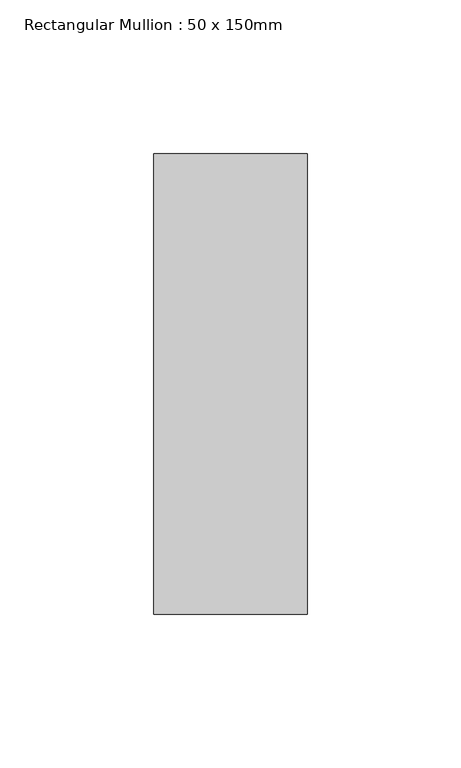
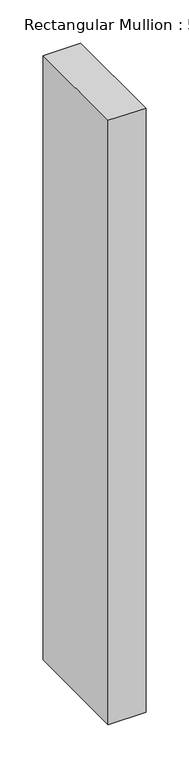
"""IFC4 building model written with IfcOpenShell, lengths in millimetres: member geometry, Rectangular Mullion : 50 x 150mm."""

from ifc_helpers import new_model, si_unit, frame, origin, place, context, project, spatial, polyline, outline, extrude, source, transform, mapped, element, save


def rectangular_mullion_50_x_150mm_324a6438(model_context):
    return source(origin(), model_context, "Body", "SweptSolid", [
        extrude(outline(polyline([(0.0, 75.0), (0.0, -75.0), (-50.0, -75.0), (-50.0, 75.0), (0.0, 75.0)])), frame((0.0, 0.0, -850.0), z_axis=(0.0, 0.0, 1.0), x_axis=(1.0, 0.0, 0.0)), (0.0, 0.0, 1.0), 850.0),
    ])


if __name__ == "__main__":
    model = new_model("IFC4")
    model_context = context("Model", 3, world=origin())
    ifc_project = project(units=[si_unit("LENGTHUNIT", "METRE", prefix="MILLI")], contexts=[model_context])
    site = spatial("IfcSite", under=ifc_project)
    building = spatial("IfcBuilding", under=site)
    placement = place(None, origin())
    rectangular_mullion_50_x_150mm_shape = rectangular_mullion_50_x_150mm_324a6438(model_context)
    element("IfcMember", 1, ObjectType="Rectangular Mullion : 50 x 150mm", at=placement, inside=building, context=model_context, shape_type="MappedRepresentation", body=[
        mapped(rectangular_mullion_50_x_150mm_shape, transform((0.0, 0.0, 0.0), x_axis=(1.0, 0.0, 0.0), y_axis=(0.0, 1.0, 0.0), z_axis=(0.0, 0.0, 1.0))),
    ])
    save(model, "model.ifc")

# Revit data of these elements
# Type "Rectangular Mullion : 50 x 150mm"
#   built-in parameter 1007304 = 0.492126 (stored number, unit not read)
#   built-in parameter 1007301 = 0.082021 (stored number, unit not read)
#   built-in parameter 1007300 = 0.082021 (stored number, unit not read)
# Element 1 (IfcMember, "Rectangular Mullion : 50 x 150mm")
#   Materials on its faces: "Aluminium"
# Materials
#   "Aluminium": class "Metal", colour RGB 247 247 247, transparency 0, Description = "Aluminium 6061", Cost = 0
